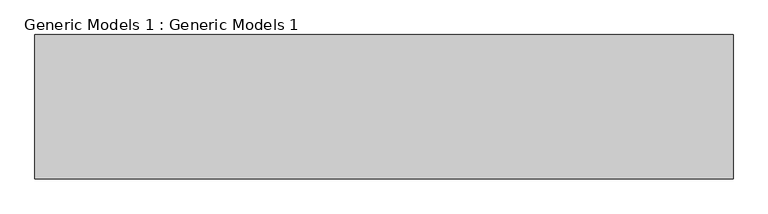
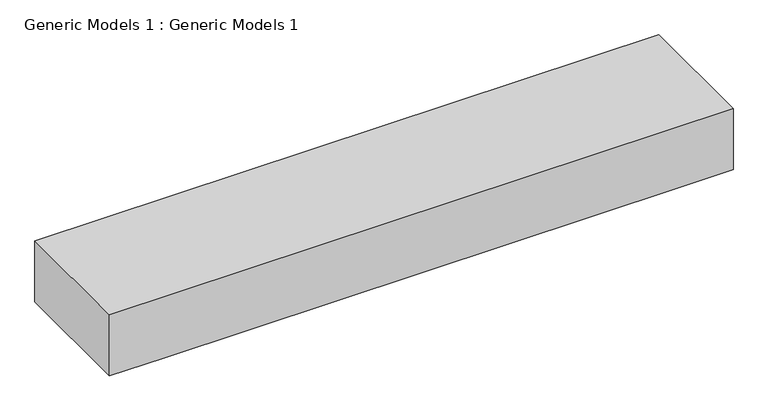
"""IFC4 building model written with IfcOpenShell, lengths in millimetres: proxy geometry, Generic Models 1 : Generic Models 1."""

from ifc_helpers import new_model, si_unit, frame, origin, place, context, project, spatial, polyline, outline, extrude, source, transform, mapped, element, save


def generic_models_1_generic_models_1_fbb7ad13(model_context):
    return source(origin(), model_context, "Body", "SweptSolid", [
        extrude(outline(polyline([(17373.6, -3917.9887202), (17373.6, -3790.9887202), (17526.0, -3790.9887202), (17526.0, -5264.1887202), (17373.6, -5264.1887202), (17373.6, -5137.1887202), (17373.6, -3917.9887202)])), frame((0.0, -3543.5690997, 0.0), z_axis=(0.0, 1.0, 0.0), x_axis=(0.0, 0.0, 1.0)), (0.0, 0.0, 1.0), 304.8),
    ])


if __name__ == "__main__":
    model = new_model("IFC4")
    model_context = context("Model", 3, world=origin())
    ifc_project = project(units=[si_unit("LENGTHUNIT", "METRE", prefix="MILLI")], contexts=[model_context])
    site = spatial("IfcSite", under=ifc_project)
    building = spatial("IfcBuilding", under=site)
    placement = place(None, origin())
    generic_models_1_generic_models_1_shape = generic_models_1_generic_models_1_fbb7ad13(model_context)
    element("IfcBuildingElementProxy", 1, Name="Generic Models 1 : Generic Models 1", ObjectType="Generic Models 1 : Generic Models 1", at=placement, inside=building, context=model_context, shape_type="MappedRepresentation", body=[
        mapped(generic_models_1_generic_models_1_shape, transform((0.0, 0.0, 0.0), x_axis=(1.0, 0.0, 0.0), y_axis=(0.0, 1.0, 0.0), z_axis=(0.0, 0.0, 1.0))),
    ])
    save(model, "model.ifc")

# Revit data of these elements
# Element 1 (IfcBuildingElementProxy, "Generic Models 1 : Generic Models 1")
#   Materials on its faces: "white"
# Materials
#   "white": class "Generic", colour RGB 120 120 120, transparency 0, Cost = 0
